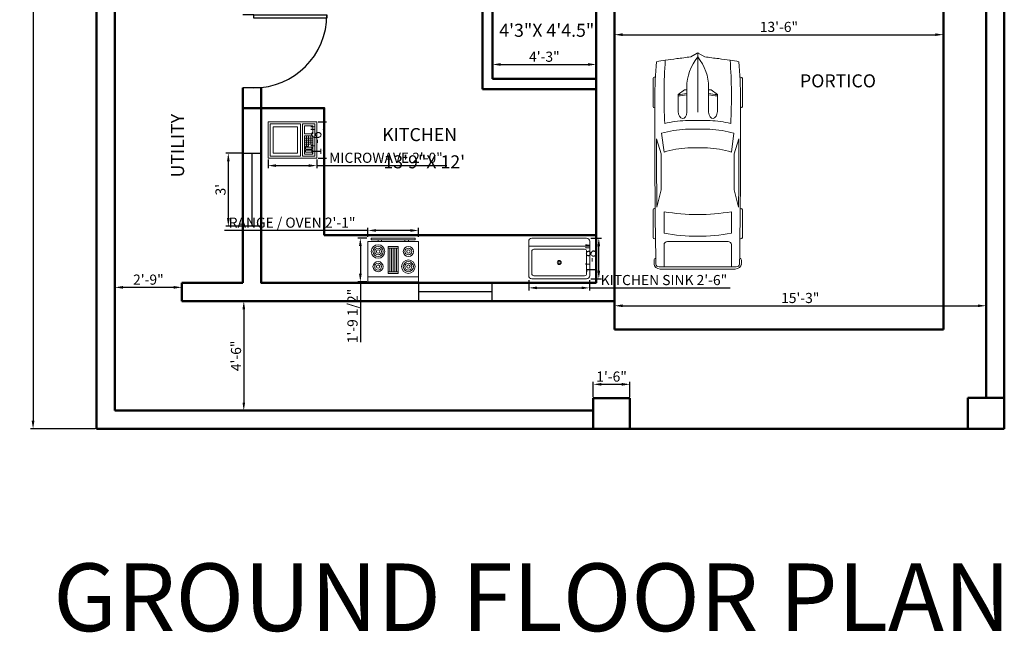
# Model space of a CAD drawing. Units: inches. Extents: x 116541 to 117938, y 135634 to 136328.
# Tile 1 of 9: x 116545 to 117030, y 135634 to 135936. Entities that reach past the tile are written whole.
import ezdxf

# ---------------------------------------------------------------- set-up
doc = ezdxf.new("R2010")
doc.units = ezdxf.units.IN
for name, color, linetype, lineweight in [('A-ANNO-DIMS', 2, 'Continuous', 18), ('A-ANNO-TEXT', 7, 'Continuous', 25), ('A-AREA-IDEN', 3, 'Continuous', 25), ('A-DOOR', 4, 'Continuous', 25), ('A-EQPM', 8, 'Continuous', 18), ('A-FLOR-FIXT', 9, 'Continuous', 18), ('A-GLAZ', 1, 'Continuous', 25), ('A-WALL', 7, 'Continuous', 50)]:
    doc.layers.add(name, color=color, linetype=linetype, lineweight=lineweight)
doc.styles.get("Standard").update_dxf_attribs({"font": 'arial.ttf'})
doc.dimstyles.new('ISO-25', dxfattribs={"dimtxt": 5, "dimasz": 4, "dimexe": 1.25, "dimexo": 0.625, "dimtad": 1, "dimdec": 3, "dimlunit": 3, "dimtxsty": 'Standard', "dimcen": 2.5, "dimadec": 0, "dimazin": 0, "dimtfac": 1, "dimtdec": 3, "dimtmove": 0, "dimatfit": 3, "dimfxl": 1, "dimarcsym": 0})

# ---------------------------------------------------------------- blocks, each defined once
blk = doc.blocks.new('*U4')
for p, q in [((-40, 0), (-40, 6)), ((0, 0), (0, 6))]:
    blk.add_line(p, q)
blk.add_lwpolyline([(0, 0), (0, -40), (-1.75, -40), (-1.75, 0)], close=True)
blk.add_arc((0, 0), 40, 180, 270)
blk = doc.blocks.new('Microwave')
for p, q in [((18, 10), (22, 10)), ((19, 7), (19, 11)), ((20, 11), (20, 7)), ((21, 7), (21, 11)), ((22, 9), (18, 9)), ((18, 8), (22, 8)), ((22, 7), (18, 7)), ((20, 6), (18, 6)), ((19, 6), (19, 7)), ((20, 7), (20, 6))]:
    blk.add_line(p, q)
for points in [[(0, 0), (0, 18), (24, 18), (24, 0)], [(1, 1), (1, 17), (16, 17), (16, 1)], [(2.5, 2.5), (2.5, 15.5), (14.5, 15.5), (14.5, 2.5)], [(17, 1), (17, 17), (23, 17), (23, 1)], [(18, 12), (18, 16), (22, 16), (22, 12)], [(18, 2), (18, 11), (22, 11), (22, 2)], [(18.5, 4.5), (18.5, 5.5), (21.5, 5.5), (21.5, 4.5)], [(18.5, 3), (18.5, 4), (21.5, 4), (21.5, 3)]]:
    blk.add_lwpolyline(points, close=True)
blk = doc.blocks.new('Range-Oven - 30 in top')
for p, q in [((0, -3), (30, -3)), ((12, -6), (18, -6)), ((13, -20), (13, -6)), ((14, -6), (14, -20)), ((15, -20), (15, -6)), ((16, -6), (16, -20)), ((17, -20), (17, -6)), ((18, -20), (12, -20)), ((6, -24), (6, -25)), ((8, -25), (8, -24)), ((22, -25), (22, -24)), ((24, -24), (24, -25))]:
    blk.add_line(p, q)
for points in [[(0, -24), (0, 0), (30, 0), (30, -24)], [(12, -21), (12, -5), (18, -5), (18, -21)], [(2, -26), (2, -25), (28, -25), (28, -26)]]:
    blk.add_lwpolyline(points, close=True)
for centre, radius in [((6, -9), 4), ((6, -9), 3), ((6, -9), 2), ((6, -9), 1), ((24, -9), 3), ((24, -9), 2), ((24, -9), 1), ((6, -18), 3), ((6, -18), 2), ((6, -18), 1), ((24, -18), 4), ((24, -18), 3), ((24, -18), 2), ((24, -18), 1)]:
    blk.add_circle(centre, radius)
blk = doc.blocks.new('Sink-single - 30 in top')
blk.add_line((-15, -3.999996), (15, -3.999996))
for points in [[(-13.5, 0), (13.5, 0)], [(-15, -18.499996), (-15, -1.5)], [(15, -1.5), (15, -18.499996)], [(-13.5, -17.499996), (-13.5, -6.499996)], [(-12.5, -5.499996), (12.5, -5.499996)], [(13.5, -6.499996), (13.5, -17.499996)], [(12.5, -18.499996), (-12.5, -18.499996)], [(13.5, -19.999996), (-13.5, -19.999996)]]:
    blk.add_lwpolyline(points)
for radius in [1, 0.5]:
    blk.add_circle((0, -11.999996), radius)
for centre, radius, start, end in [((-13.5, -1.5), 1.5, 90, 180), ((13.5, -1.5), 1.5, 0, 90), ((-12.5, -6.499996), 1, 90, 180), ((12.5, -6.499996), 1, 0, 90), ((-13.5, -18.499996), 1.5, 180, 270), ((-12.5, -17.499996), 1, 180, 270), ((12.5, -17.499996), 1, 270, 0), ((13.5, -18.499996), 1.5, 270, 0)]:
    blk.add_arc(centre, radius, start, end)
blk = doc.blocks.new('*U20')
for p, q in [((21.1, 37.41), (21.1, 36.83)), ((46.55, 38.89), (22.35, 38.89)), ((47.8, 37.39), (47.8, 37.41)), ((87.99, 31.87), (74.76, 35.92)), ((134.31, 35.6), (119.29, 31.78)), ((135.45, 37.07), (135.45, 37.41)), ((136.7, 38.89), (160.9, 38.89)), ((162.15, 37.41), (162.15, 36.77)), ((70.03, 31.54), (86.41, 29.35)), ((138.42, 29.35), (157.25, 29.35)), ((164.52, 26.39), (164.52, -26.39)), ((186.47, 29.35), (167.01, 29.35)), ((186.47, -33.5), (186.47, 33.5)), ((188.4, -32.76), (188.4, 32.76)), ((32.27, 11.63), (36.13, 17.17)), ((36.13, 17.17), (50.94, 17.17)), ((29.77, 9.51), (51.68, 9.51)), ((32.12, 9.51), (32.12, 11.15)), ((58.92, -10.77), (58.92, 10.77)), ((66.55, -10.53), (66.55, 10.53)), ((186.47, -10.53), (186.47, 10.53)), ((3.27, 6.13), (0.1, 0.41)), ((82.74, 8.5), (82.74, -8.5)), ((0, 0), (51.68, 0)), ((0.1, -0.41), (3.27, -6.13)), ((29.77, -9.51), (51.68, -9.51)), ((32.12, -9.51), (32.12, -11.15)), ((32.27, -11.63), (36.13, -17.17)), ((36.13, -17.17), (50.94, -17.17)), ((86.41, -29.35), (70.03, -31.54)), ((87.99, -31.87), (74.76, -35.92)), ((134.31, -35.6), (119.29, -31.78)), ((157.25, -29.35), (138.42, -29.35)), ((167.01, -29.35), (186.47, -29.35)), ((21.1, -37.41), (21.1, -36.83)), ((46.55, -38.89), (22.35, -38.89)), ((47.8, -37.39), (47.8, -37.41)), ((135.45, -37.07), (135.45, -37.41)), ((136.7, -38.89), (160.9, -38.89)), ((162.15, -37.41), (162.15, -36.77))]:
    blk.add_line(p, q)
for centre, major_axis, ratio, start_param, end_param in [((266.03, -27.52), (0, 313.31), 0.842304, 1.367076, 1.39176), ((41.19, -490.86), (0, 528.23), 0.842304, 0.00281, 0.075598), ((22.35, 37.41), (0, -1.48), 0.842304, 3.141593, 4.712389), ((64.48, -10555.62), (0, 10593.03), 0.842304, -0.013397, 0.002797), ((46.55, 37.41), (0, 1.48), 0.842304, -1.570796, 0), ((64.48, -10555.62), (0, -10591.55), 0.842304, 3.133765, 3.140441), ((136.7, 37.41), (0, -1.48), 0.842304, 3.141593, 4.712389), ((160.9, 37.41), (0, 1.48), 0.842304, -1.570796, 0), ((180.63, 35.84), (0, 2.22), 0.842304, -0.013017, 1.249894), ((64.48, -10556.36), (0, 10595.31), 0.842304, -0.013397, -0.013017), ((183.98, 33.5), (0, -2.96), 0.842304, 1.570796, 3.128196), ((183.98, 32.76), (0, -5.25), 0.842304, 1.570796, 3.128196), ((259.18, -27.52), (0, -305.3), 0.842304, 4.528606, 4.561838), ((37.47, -593.96), (0, -623.33), 0.842304, 3.096046, 3.200911), ((134.4, 5.39), (0, -89.78), 0.842304, 4.449482, 4.652344), ((135.29, 5.39), (0, 81.77), 0.842304, 1.245306, 1.50788), ((149.6, 2.8), (0, -79.58), 0.842304, 4.372215, 4.640744), ((95.79, -3666.35), (0, -3698.24), 0.842304, 3.134049, 3.144098), ((17.08, 0), (0, 147.02), 0.842304, 4.511394, 4.913384), ((35.91, 0), (0, 147.02), 0.842304, 4.511394, 4.913384), ((167.01, 26.39), (0, 2.96), 0.842304, 0, 1.570796), ((-204.49, 52.4), (0, -250.96), 0.842304, 1.385369, 1.434372), ((13.04, 17.01), (0, 27.42), 0.842304, 4.435146, 4.718221), ((14.2, 17.01), (0, 27.42), 0.842304, 4.435146, 4.718221), ((50.79, 13.34), (6.34, -0.36), 0.603834, -1.395552, 1.581315), ((29.77, -46.66), (0, 56.17), 0.842304, 0, 0.590319), ((32.75, 11.15), (0, 0.74), 0.842304, 0.879714, 1.570796), ((0.62, 0), (0, -0.74), 0.842304, 4.131459, 5.293319), ((-204.49, -52.4), (0, 250.96), 0.842304, -1.434372, -1.385369), ((29.77, 46.66), (0, 56.17), 0.842304, 2.551274, 3.141593), ((149.6, -2.8), (0, -79.58), 0.842304, -1.499151, -1.230623), ((32.75, -11.15), (0, -0.74), 0.842304, 4.712389, 5.403472), ((13.04, -17.01), (0, -27.42), 0.842304, 1.564964, 1.848039), ((14.2, -17.01), (0, -27.42), 0.842304, 1.564964, 1.848039), ((134.4, -5.39), (0, -89.78), 0.842304, -1.510751, -1.307889), ((135.29, -5.39), (0, -81.77), 0.842304, -1.50788, -1.245306), ((259.18, 27.52), (0, 305.3), 0.842304, 1.721348, 1.754579), ((266.03, 27.52), (0, 313.31), 0.842304, 1.749832, 1.774517), ((37.47, 593.96), (0, -623.33), 0.842304, -0.059319, 0.045547), ((95.79, 3666.35), (0, -3698.24), 0.842304, -0.002505, 0.007544), ((167.01, -26.39), (0, -2.96), 0.842304, 4.712389, 6.283185), ((183.98, -33.5), (0, 2.96), 0.842304, 3.15499, 4.712389), ((183.98, -32.76), (0, -5.25), 0.842304, 0.013397, 1.570796), ((41.19, 490.86), (0, -528.23), 0.842304, -0.075598, -0.00281), ((22.35, -37.41), (0, 1.48), 0.842304, 1.570796, 3.141593), ((64.48, 10555.62), (0, 10593.03), 0.842304, 3.138796, 3.15499), ((46.55, -37.41), (0, -1.48), 0.842304, 0, 1.570796), ((64.48, 10555.62), (0, -10591.55), 0.842304, 0.001152, 0.007828), ((136.7, -37.41), (0, -1.48), 0.842304, -1.570796, 0), ((160.9, -37.41), (0, 1.48), 0.842304, 3.141593, 4.712389), ((180.63, -35.84), (0, -2.22), 0.842304, -1.249894, 0.013017), ((64.48, 10556.36), (0, 10595.31), 0.842304, 3.15461, 3.15499)]:
    blk.add_ellipse(centre, major_axis=major_axis, ratio=ratio, start_param=start_param, end_param=end_param)
at = {"extrusion": (0, 0, -1)}
blk.add_ellipse((50.79, -13.34), major_axis=(6.34, 0.36), ratio=0.603834, start_param=-1.395552, end_param=1.581315, dxfattribs=at)
blk = doc.blocks.new('*D21')
at = {"layer": 'A-ANNO-DIMS', "color": 0, "lineweight": -2, "transparency": 16777216}
for p, q in [((116592.18, 135805.88), (116592.18, 135803.01)), ((116625.18, 135805.88), (116625.18, 135803.01)), ((116621.18, 135804.26), (116596.18, 135804.26))]:
    blk.add_line(p, q, dxfattribs=at)
at = {"layer": 'A-ANNO-DIMS', "color": 0, "transparency": 16777216}
for points in [[(116596.18, 135804.92), (116596.18, 135803.59), (116592.18, 135804.26)], [(116621.18, 135804.92), (116621.18, 135803.59), (116625.18, 135804.26)]]:
    blk.add_solid(points, dxfattribs=at)
at = {"layer": 'Defpoints', "color": 0, "transparency": 16777216}
for p in [(116592.18, 135806.5), (116625.18, 135806.5), (116592.18, 135804.26)]:
    blk.add_point(p, dxfattribs=at)
at = {"layer": 'A-ANNO-DIMS', "color": 0, "transparency": 16777216, "insert": (116608.68, 135807.43), "char_height": 5, "attachment_point": 5}
blk.add_mtext('2\'-9"', dxfattribs=at)
blk = doc.blocks.new('*D22')
at = {"layer": 'A-ANNO-DIMS', "color": 0, "lineweight": -2, "transparency": 16777216}
for p, q in [((116655.06, 135797.5), (116654.42, 135797.5)), ((116655.67, 135793.5), (116655.67, 135747.5)), ((116655.06, 135743.5), (116654.42, 135743.5))]:
    blk.add_line(p, q, dxfattribs=at)
at = {"layer": 'A-ANNO-DIMS', "color": 0, "transparency": 16777216}
for points in [[(116655.01, 135793.5), (116656.34, 135793.5), (116655.67, 135797.5)], [(116655.01, 135747.5), (116656.34, 135747.5), (116655.67, 135743.5)]]:
    blk.add_solid(points, dxfattribs=at)
at = {"layer": 'Defpoints', "color": 0, "transparency": 16777216}
for p in [(116655.68, 135797.5), (116655.67, 135743.5), (116655.68, 135743.5)]:
    blk.add_point(p, dxfattribs=at)
at = {"layer": 'A-ANNO-DIMS', "color": 0, "transparency": 16777216, "insert": (116652.49, 135770.5), "char_height": 5, "attachment_point": 5, "rotation": 90}
blk.add_mtext('4\'-6"', dxfattribs=at)
blk = doc.blocks.new('*D23')
at = {"layer": 'A-ANNO-DIMS', "color": 0, "lineweight": -2, "transparency": 16777216}
for p, q in [((116778.18, 135907.63), (116778.18, 135915.36)), ((116782.18, 135914.11), (116825.18, 135914.11)), ((116829.18, 135907.63), (116829.18, 135915.36))]:
    blk.add_line(p, q, dxfattribs=at)
at = {"layer": 'A-ANNO-DIMS', "color": 0, "transparency": 16777216}
for points in [[(116782.18, 135914.77), (116782.18, 135913.44), (116778.18, 135914.11)], [(116825.18, 135914.77), (116825.18, 135913.44), (116829.18, 135914.11)]]:
    blk.add_solid(points, dxfattribs=at)
at = {"layer": 'Defpoints', "color": 0, "transparency": 16777216}
for p in [(116829.18, 135914.11), (116778.18, 135907), (116829.18, 135907)]:
    blk.add_point(p, dxfattribs=at)
at = {"layer": 'A-ANNO-DIMS', "color": 0, "transparency": 16777216, "insert": (116803.68, 135917.29), "char_height": 5, "attachment_point": 5}
blk.add_mtext('4\'-3"', dxfattribs=at)
blk = doc.blocks.new('*D24')
at = {"layer": 'A-ANNO-DIMS', "color": 0, "lineweight": -2, "transparency": 16777216}
for p, q in [((116838.18, 135920.77), (116838.18, 135930.04)), ((116842.18, 135928.79), (116996.18, 135928.79)), ((117000.18, 135920.77), (117000.18, 135930.04))]:
    blk.add_line(p, q, dxfattribs=at)
at = {"layer": 'A-ANNO-DIMS', "color": 0, "transparency": 16777216}
for points in [[(116842.18, 135929.46), (116842.18, 135928.13), (116838.18, 135928.79)], [(116996.18, 135929.46), (116996.18, 135928.13), (117000.18, 135928.79)]]:
    blk.add_solid(points, dxfattribs=at)
at = {"layer": 'Defpoints', "color": 0, "transparency": 16777216}
for p in [(117000.18, 135928.79), (116838.18, 135920.14), (117000.18, 135920.14)]:
    blk.add_point(p, dxfattribs=at)
at = {"layer": 'A-ANNO-DIMS', "color": 0, "transparency": 16777216, "insert": (116919.18, 135931.97), "char_height": 5, "attachment_point": 5}
blk.add_mtext('13\'-6"', dxfattribs=at)
blk = doc.blocks.new('*D25')
at = {"layer": 'A-ANNO-DIMS', "color": 0, "lineweight": -2, "transparency": 16777216}
for p, q in [((116838.18, 135796.88), (116838.18, 135793.95)), ((117021.18, 135795.82), (117021.18, 135796.45)), ((116842.18, 135795.2), (117017.18, 135795.2))]:
    blk.add_line(p, q, dxfattribs=at)
at = {"layer": 'A-ANNO-DIMS', "color": 0, "transparency": 16777216}
for points in [[(116842.18, 135795.86), (116842.18, 135794.53), (116838.18, 135795.2)], [(117017.18, 135795.86), (117017.18, 135794.53), (117021.18, 135795.2)]]:
    blk.add_solid(points, dxfattribs=at)
at = {"layer": 'Defpoints', "color": 0, "transparency": 16777216}
for p in [(116838.18, 135797.5), (117021.18, 135795.2), (117021.18, 135795.2)]:
    blk.add_point(p, dxfattribs=at)
at = {"layer": 'A-ANNO-DIMS', "color": 0, "transparency": 16777216, "insert": (116929.68, 135798.38), "char_height": 5, "attachment_point": 5}
blk.add_mtext('15\'-3"', dxfattribs=at)
blk = doc.blocks.new('*D26')
at = {"layer": 'A-ANNO-DIMS', "color": 0, "lineweight": -2, "transparency": 16777216}
for p, q in [((116582.55, 136286.5), (116550.65, 136286.5)), ((116551.9, 136282.5), (116551.9, 135738.5)), ((116582.55, 135734.5), (116550.65, 135734.5))]:
    blk.add_line(p, q, dxfattribs=at)
at = {"layer": 'A-ANNO-DIMS', "color": 0, "transparency": 16777216}
for points in [[(116551.23, 136282.5), (116552.56, 136282.5), (116551.9, 136286.5)], [(116551.23, 135738.5), (116552.56, 135738.5), (116551.9, 135734.5)]]:
    blk.add_solid(points, dxfattribs=at)
at = {"layer": 'Defpoints', "color": 0, "transparency": 16777216}
for p in [(116583.18, 136286.5), (116551.9, 135734.5), (116583.18, 135734.5)]:
    blk.add_point(p, dxfattribs=at)
at = {"layer": 'A-ANNO-DIMS', "color": 0, "transparency": 16777216, "insert": (116548.72, 136010.5), "char_height": 5, "attachment_point": 5, "rotation": 90}
blk.add_mtext("46'", dxfattribs=at)
blk = doc.blocks.new('*D33')
at = {"layer": 'A-ANNO-DIMS', "color": 0, "lineweight": -2, "transparency": 16777216}
for p, q in [((116654.55, 135870.39), (116646.8, 135870.39)), ((116648.05, 135866.39), (116648.05, 135838.39)), ((116654.55, 135834.39), (116646.8, 135834.39))]:
    blk.add_line(p, q, dxfattribs=at)
at = {"layer": 'A-ANNO-DIMS', "color": 0, "transparency": 16777216}
for points in [[(116647.39, 135866.39), (116648.72, 135866.39), (116648.05, 135870.39)], [(116647.39, 135838.39), (116648.72, 135838.39), (116648.05, 135834.39)]]:
    blk.add_solid(points, dxfattribs=at)
at = {"layer": 'Defpoints', "color": 0, "transparency": 16777216}
for p in [(116655.18, 135870.39), (116648.05, 135834.39), (116655.18, 135834.39)]:
    blk.add_point(p, dxfattribs=at)
at = {"layer": 'A-ANNO-DIMS', "color": 0, "transparency": 16777216, "insert": (116644.87, 135852.39), "char_height": 5, "attachment_point": 5, "rotation": 90}
blk.add_mtext("3'", dxfattribs=at)
blk = doc.blocks.new('*D35')
at = {"layer": 'A-ANNO-DIMS', "color": 0, "lineweight": -2, "transparency": 16777216}
for p, q in [((116827.78, 135750.2), (116827.78, 135757.72)), ((116845.78, 135750.2), (116845.78, 135757.72)), ((116841.78, 135756.47), (116831.78, 135756.47))]:
    blk.add_line(p, q, dxfattribs=at)
at = {"layer": 'A-ANNO-DIMS', "color": 0, "transparency": 16777216}
for points in [[(116831.78, 135757.14), (116831.78, 135755.8), (116827.78, 135756.47)], [(116841.78, 135757.14), (116841.78, 135755.8), (116845.78, 135756.47)]]:
    blk.add_solid(points, dxfattribs=at)
at = {"layer": 'Defpoints', "color": 0, "transparency": 16777216}
for p in [(116827.78, 135756.47), (116827.78, 135749.57), (116845.78, 135749.57)]:
    blk.add_point(p, dxfattribs=at)
at = {"layer": 'A-ANNO-DIMS', "color": 0, "transparency": 16777216, "insert": (116836.78, 135759.65), "char_height": 5, "attachment_point": 5}
blk.add_mtext('1\'-6"', dxfattribs=at)
blk = doc.blocks.new('*D84')
at = {"layer": 'A-ANNO-DIMS', "color": 0, "lineweight": -2, "transparency": 16777216}
for p, q in [((116667.6, 135867.24), (116667.6, 135863.02)), ((116671.6, 135864.27), (116687.6, 135864.27)), ((116691.6, 135867.24), (116691.6, 135863.02)), ((116691.6, 135864.27), (116755.71, 135864.27))]:
    blk.add_line(p, q, dxfattribs=at)
at = {"layer": 'A-ANNO-DIMS', "color": 0, "transparency": 16777216}
for points in [[(116671.6, 135864.93), (116671.6, 135863.6), (116667.6, 135864.27)], [(116687.6, 135864.93), (116687.6, 135863.6), (116691.6, 135864.27)]]:
    blk.add_solid(points, dxfattribs=at)
at = {"layer": 'Defpoints', "color": 0, "transparency": 16777216}
for p in [(116667.6, 135867.87), (116691.6, 135867.87), (116691.6, 135864.27)]:
    blk.add_point(p, dxfattribs=at)
at = {"layer": 'A-ANNO-DIMS', "color": 0, "transparency": 16777216, "insert": (116725.66, 135867.48), "char_height": 5, "attachment_point": 5}
blk.add_mtext('MICROWAVE 2\'-0"', dxfattribs=at)
blk = doc.blocks.new('*D85')
at = {"layer": 'A-ANNO-DIMS', "color": 0, "lineweight": -2, "transparency": 16777216}
for p, q in [((116692.23, 135885.87), (116696.45, 135885.87)), ((116695.2, 135871.87), (116695.2, 135881.87)), ((116692.23, 135867.87), (116696.45, 135867.87))]:
    blk.add_line(p, q, dxfattribs=at)
at = {"layer": 'A-ANNO-DIMS', "color": 0, "transparency": 16777216}
for points in [[(116694.54, 135881.87), (116695.87, 135881.87), (116695.2, 135885.87)], [(116694.54, 135871.87), (116695.87, 135871.87), (116695.2, 135867.87)]]:
    blk.add_solid(points, dxfattribs=at)
at = {"layer": 'Defpoints', "color": 0, "transparency": 16777216}
for p in [(116691.6, 135885.87), (116695.2, 135885.87), (116691.6, 135867.87)]:
    blk.add_point(p, dxfattribs=at)
at = {"layer": 'A-ANNO-DIMS', "color": 0, "transparency": 16777216, "insert": (116692.03, 135876.87), "char_height": 5, "attachment_point": 5, "rotation": 90}
blk.add_mtext('1\'-6"', dxfattribs=at)
blk = doc.blocks.new('*D86')
at = {"layer": 'A-ANNO-DIMS', "color": 0, "lineweight": -2, "transparency": 16777216}
for p, q in [((116716.8, 135832.31), (116646.12, 135832.31)), ((116716.8, 135829.2), (116716.8, 135833.56)), ((116737.69, 135832.31), (116720.8, 135832.31)), ((116741.69, 135829.2), (116741.69, 135833.56))]:
    blk.add_line(p, q, dxfattribs=at)
at = {"layer": 'A-ANNO-DIMS', "color": 0, "transparency": 16777216}
for points in [[(116720.8, 135832.98), (116720.8, 135831.64), (116716.8, 135832.31)], [(116737.69, 135832.98), (116737.69, 135831.64), (116741.69, 135832.31)]]:
    blk.add_solid(points, dxfattribs=at)
at = {"layer": 'Defpoints', "color": 0, "transparency": 16777216}
for p in [(116716.8, 135832.31), (116716.8, 135828.58), (116741.69, 135828.58)]:
    blk.add_point(p, dxfattribs=at)
at = {"layer": 'A-ANNO-DIMS', "color": 0, "transparency": 16777216, "insert": (116679.46, 135835.52), "char_height": 5, "attachment_point": 5}
blk.add_mtext('RANGE / OVEN 2\'-1"', dxfattribs=at)
blk = doc.blocks.new('*D87')
at = {"layer": 'A-ANNO-DIMS', "color": 0, "lineweight": -2, "transparency": 16777216}
for p, q in [((116716.18, 135828.58), (116711.82, 135828.58)), ((116713.07, 135824.58), (116713.07, 135811.01)), ((116716.18, 135807.01), (116711.82, 135807.01)), ((116713.07, 135807.01), (116713.07, 135777.29))]:
    blk.add_line(p, q, dxfattribs=at)
at = {"layer": 'A-ANNO-DIMS', "color": 0, "transparency": 16777216}
for points in [[(116712.4, 135824.58), (116713.74, 135824.58), (116713.07, 135828.58)], [(116712.4, 135811.01), (116713.74, 135811.01), (116713.07, 135807.01)]]:
    blk.add_solid(points, dxfattribs=at)
at = {"layer": 'Defpoints', "color": 0, "transparency": 16777216}
for p in [(116716.8, 135828.58), (116713.07, 135807.01), (116716.8, 135807.01)]:
    blk.add_point(p, dxfattribs=at)
at = {"layer": 'A-ANNO-DIMS', "color": 0, "transparency": 16777216, "insert": (116709.86, 135790.15), "char_height": 5, "attachment_point": 5, "rotation": 90}
blk.add_mtext('1\'-9 1/2"', dxfattribs=at)
blk = doc.blocks.new('*D94')
at = {"layer": 'A-ANNO-DIMS', "color": 0, "lineweight": -2, "transparency": 16777216}
for p, q in [((116795.99, 135807.89), (116795.99, 135802.76)), ((116825.99, 135807.89), (116825.99, 135802.76)), ((116799.99, 135804.01), (116821.99, 135804.01)), ((116825.99, 135804.01), (116895.16, 135804.01))]:
    blk.add_line(p, q, dxfattribs=at)
at = {"layer": 'A-ANNO-DIMS', "color": 0, "transparency": 16777216}
for points in [[(116799.99, 135804.68), (116799.99, 135803.35), (116795.99, 135804.01)], [(116821.99, 135804.68), (116821.99, 135803.35), (116825.99, 135804.01)]]:
    blk.add_solid(points, dxfattribs=at)
at = {"layer": 'Defpoints', "color": 0, "transparency": 16777216}
for p in [(116795.99, 135808.51), (116825.99, 135808.51), (116825.99, 135804.01)]:
    blk.add_point(p, dxfattribs=at)
at = {"layer": 'A-ANNO-DIMS', "color": 0, "transparency": 16777216, "insert": (116862.58, 135807.22), "char_height": 5, "attachment_point": 5}
blk.add_mtext('KITCHEN SINK 2\'-6"', dxfattribs=at)
blk = doc.blocks.new('*D95')
at = {"layer": 'A-ANNO-DIMS', "color": 0, "lineweight": -2, "transparency": 16777216}
for p, q in [((116826.62, 135828.51), (116831.74, 135828.51)), ((116830.49, 135812.51), (116830.49, 135824.51)), ((116826.62, 135808.51), (116831.74, 135808.51))]:
    blk.add_line(p, q, dxfattribs=at)
at = {"layer": 'A-ANNO-DIMS', "color": 0, "transparency": 16777216}
for points in [[(116829.83, 135824.51), (116831.16, 135824.51), (116830.49, 135828.51)], [(116829.83, 135812.51), (116831.16, 135812.51), (116830.49, 135808.51)]]:
    blk.add_solid(points, dxfattribs=at)
at = {"layer": 'Defpoints', "color": 0, "transparency": 16777216}
for p in [(116825.99, 135828.51), (116830.49, 135828.51), (116825.99, 135808.51)]:
    blk.add_point(p, dxfattribs=at)
at = {"layer": 'A-ANNO-DIMS', "color": 0, "transparency": 16777216, "insert": (116827.32, 135818.51), "char_height": 5, "attachment_point": 5, "rotation": 90}
blk.add_mtext('1\'-8"', dxfattribs=at)

msp = doc.modelspace()

# ---------------------------------------------------------------- linework, layer by layer
at = {"layer": 'A-DOOR'}
msp.add_lwpolyline([(116664.1763, 135902.7493), (116664.1763, 135902.5688), (116655.1763, 135902.5688)], dxfattribs=at)
at = {"layer": 'A-GLAZ'}
for p, q in [((116659.6763, 135870.3918), (116659.6763, 135834.3918)), ((116777.7949, 135802.0034), (116741.7949, 135802.0034))]:
    msp.add_line(p, q, dxfattribs=at)
for points in [[(116655.1763, 135870.3918), (116664.1763, 135870.3918), (116664.1763, 135834.3918), (116655.1763, 135834.3918)], [(116777.7949, 135806.5034), (116777.7949, 135797.5034), (116741.7949, 135797.5034), (116741.7949, 135806.5034)]]:
    msp.add_lwpolyline(points, close=True, dxfattribs=at)
at = {"layer": 'A-WALL'}
for p, q in [((116583.1763, 136286.5034), (116583.1763, 135734.5034)), ((117030.1763, 136286.5034), (117030.1763, 135734.5034)), ((116592.1763, 136277.5034), (116592.1763, 135743.5034)), ((117021.1763, 136244.5034), (117021.1763, 135750.0323)), ((116773.1763, 135955.5034), (116773.1763, 135902.0034)), ((116778.1763, 135955.5034), (116778.1763, 135907.0034)), ((116829.1763, 135955.5034), (116829.1763, 135806.5034)), ((117000.1763, 135955.5034), (117000.1763, 135783.5034)), ((116838.1763, 135950.5034), (116838.1763, 135783.5034)), ((116664.1763, 135806.5034), (116664.1763, 135902.7493)), ((116778.1763, 135907.0034), (116829.1763, 135907.0034)), ((116655.1763, 135806.5034), (116655.1763, 135902.5688)), ((116773.1763, 135902.0034), (116829.1763, 135902.0034)), ((116664.1763, 135892.6396), (116655.1763, 135892.6396)), ((116655.1763, 135806.5034), (116625.1763, 135806.5034)), ((116625.1763, 135797.5034), (116625.1763, 135806.5034)), ((116664.1763, 135806.5034), (116829.1763, 135806.5034)), ((116625.1763, 135797.5034), (116838.1763, 135797.5034)), ((116978.7496, 135783.5034), (116838.1763, 135783.5034)), ((116978.7496, 135783.5034), (117000.1763, 135783.5034)), ((116827.7761, 135734.5034), (116827.7761, 135749.574)), ((116827.7761, 135749.574), (116845.7761, 135749.574)), ((116845.7761, 135749.574), (116845.7761, 135734.5034)), ((117030.1763, 135749.8588), (117012.1763, 135749.8588)), ((117012.1763, 135749.8588), (117012.1763, 135734.5034)), ((117030.1763, 135734.5034), (117030.1763, 135749.8588)), ((116592.1763, 135743.5034), (116827.1532, 135743.5034)), ((116583.1763, 135734.5034), (117000.1763, 135734.5034)), ((117000.1763, 135734.5034), (117030.1763, 135734.5034))]:
    msp.add_line(p, q, dxfattribs=at)
for points in [[(116695.2861, 135830.0322), (116695.2861, 135892.6396), (116664.1763, 135892.6396), (116664.1763, 135806.5034), (116695.2861, 135806.5034)], [(116695.2861, 135830.0322), (116829.1763, 135830.0322), (116829.1763, 135806.5034), (116664.1763, 135806.5034), (116664.1763, 135830.0322)]]:
    msp.add_lwpolyline(points, dxfattribs=at)

# ---------------------------------------------------------------- block references
at = {"layer": 'A-DOOR', "xscale": 0.9, "yscale": 0.9, "zscale": 0.9, "rotation": 90}
msp.add_blockref('*U4', (116660.5763, 135938.5688), dxfattribs=at)
at = {"layer": 'A-EQPM', "xscale": 0.565142980876141, "yscale": 0.565142980876141, "zscale": 0.565142980876141, "rotation": 270}
msp.add_blockref('*U20', (116879.1975, 135919.7661), dxfattribs=at)
at = {"layer": 'A-FLOR-FIXT'}
for name, p in [('Microwave', (116667.603, 135867.8656)), ('Sink-single - 30 in top', (116810.9944, 135828.5134))]:
    msp.add_blockref(name, p, dxfattribs=at)
at = {"layer": 'A-FLOR-FIXT', "xscale": 0.8295453143740938, "yscale": 0.8295453143740938, "zscale": 0.8295453143740938, "rotation": 180}
msp.add_blockref('Range-Oven - 30 in top', (116741.6882, 135807.008), dxfattribs=at)

# ---------------------------------------------------------------- texts
at = {"layer": 'A-ANNO-TEXT'}
msp.add_text('GROUND FLOOR PLAN', height=33.340721, dxfattribs=at).set_placement((116561.8257, 135634.8462))
at = {"layer": 'A-AREA-IDEN'}
for s, height, p in [('4\'3"X 4\'4.5"', 6.408368, (116781.464, 135927.7482)), ('PORTICO', 6.40837, (116929.5518, 135902.8348)), ('KITCHEN', 6.40837, (116723.8266, 135876.3457)), ('13\'9"X 12\'', 6.40837, (116724.4254, 135862.9221))]:
    msp.add_text(s, height=height, dxfattribs=at).set_placement(p)
msp.add_text('UTILITY', height=6.40837, rotation=90, dxfattribs=at).set_placement((116626.2727, 135858.4612))

# ---------------------------------------------------------------- dimensions: what is measured, and where the dimension line sits
at = {"layer": 'A-ANNO-DIMS'}
for base, p1, p2, angle, override, picture, middle in [((116551.8967, 135734.5034), (116583.1763, 136286.5034), (116583.1763, 135734.5034), 90, {"dimclrd": 0, "dimclre": 0, "dimclrt": 0}, '*D26', (116548.7188, 136010.5034)), ((116695.203, 135885.8656), (116691.603, 135867.8656), (116691.603, 135885.8656), 90, {"dimdec": 1, "dimrnd": 0, "dimzin": 1, "dimlunit": 4, "dimfrac": 2}, '*D85', (116692.0252, 135876.8656)), ((116648.0525, 135834.3918), (116655.1763, 135870.3918), (116655.1763, 135834.3918), 90, {"dimclrd": 0, "dimclre": 0, "dimclrt": 0}, '*D33', (116644.873, 135852.3918)), ((116713.0688, 135807.008), (116716.8018, 135828.5762), (116716.8018, 135807.008), 270, {"dimdec": 1, "dimrnd": 0, "dimzin": 1, "dimlunit": 4, "dimfrac": 2}, '*D87', (116709.8586, 135790.1473)), ((116830.4944, 135828.5134), (116825.9944, 135808.5134), (116825.9944, 135828.5134), 90, {"dimdec": 1, "dimrnd": 0, "dimzin": 1, "dimlunit": 4, "dimfrac": 2}, '*D95', (116827.3165, 135818.5134)), ((116655.6719, 135743.5034), (116655.6823, 135797.5034), (116655.6823, 135743.5034), 90, {"dimclrd": 0, "dimclre": 0, "dimclrt": 0}, '*D22', (116652.494, 135770.5034))]:
    dim = msp.add_linear_dim(base=base, p1=p1, p2=p2, angle=angle, dimstyle='ISO-25', override=override, dxfattribs=at)
    dim.commit()
    dim.dimension.update_dxf_attribs({"geometry": picture, "text_midpoint": middle})
for base, p1, p2, picture, middle in [((117000.1763, 135928.7918), (116838.1763, 135920.1424), (117000.1763, 135920.1424), '*D24', (116919.1763, 135931.9713)), ((116829.1763, 135914.1058), (116778.1763, 135907.0034), (116829.1763, 135907.0034), '*D23', (116803.6763, 135917.2854)), ((116592.1763, 135804.2551), (116625.1763, 135806.5034), (116592.1763, 135806.5034), '*D21', (116608.6763, 135807.4329)), ((117021.1763, 135795.1973), (116838.1763, 135797.5034), (117021.1763, 135795.1973), '*D25', (116929.6763, 135798.3769)), ((116827.7761, 135756.4687), (116845.7761, 135749.574), (116827.7761, 135749.574), '*D35', (116836.7761, 135759.6466))]:
    dim = msp.add_linear_dim(base=base, p1=p1, p2=p2, dimstyle='ISO-25', override={"dimclrd": 0, "dimclre": 0, "dimclrt": 0}, dxfattribs=at)
    dim.commit()
    dim.dimension.update_dxf_attribs({"geometry": picture, "text_midpoint": middle})
for base, p1, p2, text, picture, middle in [((116691.603, 135864.2656), (116667.603, 135867.8656), (116691.603, 135867.8656), 'MICROWAVE <>', '*D84', (116725.655, 135867.4776)), ((116825.9944, 135804.0134), (116795.9944, 135808.5134), (116825.9944, 135808.5134), 'KITCHEN SINK <>', '*D94', (116862.5754, 135807.2237))]:
    dim = msp.add_linear_dim(base=base, p1=p1, p2=p2, text=text, dimstyle='ISO-25', override={"dimdec": 1, "dimrnd": 0, "dimzin": 1, "dimlunit": 4, "dimfrac": 2}, dxfattribs=at)
    dim.commit()
    dim.dimension.update_dxf_attribs({"geometry": picture, "text_midpoint": middle})
dim = msp.add_linear_dim(base=(116716.8018, 135832.3091), p1=(116741.6882, 135828.5762), p2=(116716.8018, 135828.5762), angle=180, text='RANGE / OVEN <>', dimstyle='ISO-25', override={"dimdec": 1, "dimrnd": 0, "dimzin": 1, "dimlunit": 4, "dimfrac": 2}, dxfattribs=at)
dim.commit()
dim.dimension.update_dxf_attribs({"geometry": '*D86', "text_midpoint": (116679.4619, 135835.5211)})

doc.saveas('drawing.dxf')
